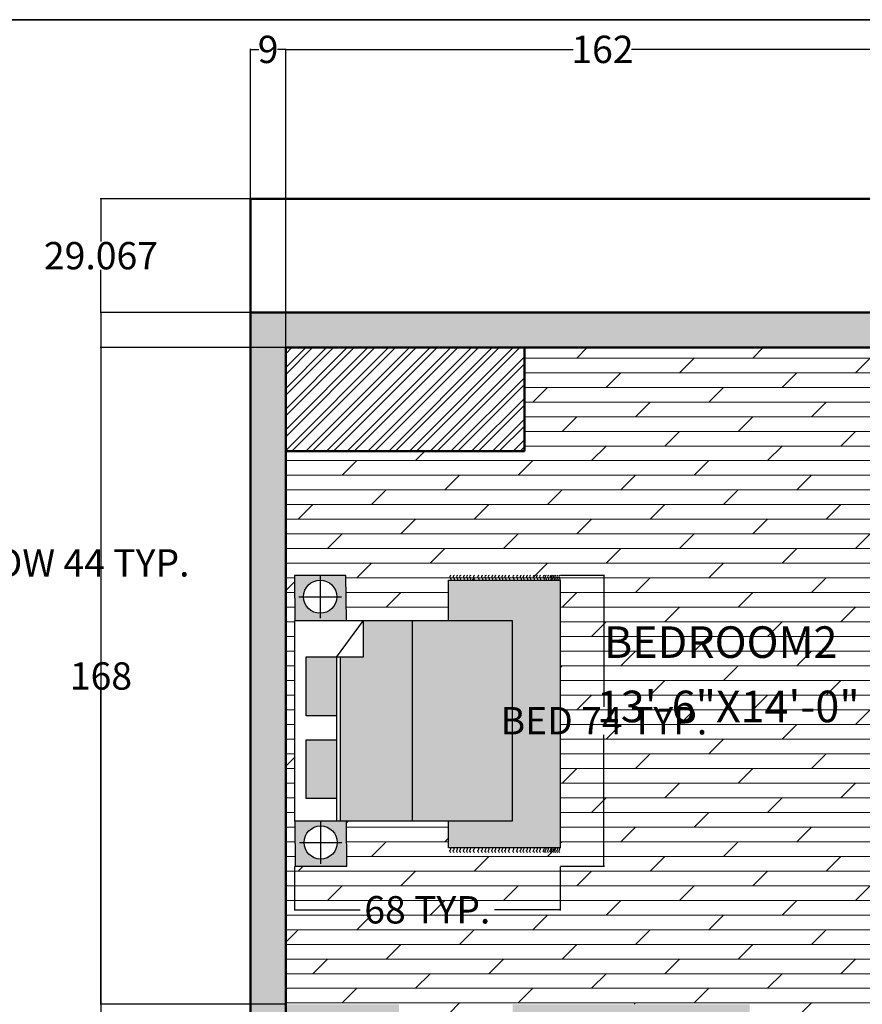
# Model space of a CAD drawing. Units: inches. Extents: x 1381 to 2246, y 1317 to 2168.
# Tile 14 of 15: x 1804 to 2019, y 1916 to 2168. Entities that reach past the tile are written whole.
import ezdxf

# ---------------------------------------------------------------- set-up
doc = ezdxf.new("R2010")
doc.units = ezdxf.units.IN
doc.header["$MEASUREMENT"] = 0
for name, color, linetype, lineweight in [('A-ANNO-DIMS', 2, 'Continuous', 18), ('A-ANNO-TTLB', 7, 'Continuous', 35), ('A-AREA-IDEN', 3, 'Continuous', 25), ('A-FLOR-PATT', 252, 'Continuous', 13), ('A-FURN', 8, 'Continuous', 18), ('A-WALL', 7, 'Continuous', 50), ('A-WALL-PATT', 8, 'Continuous', 13)]:
    doc.layers.add(name, color=color, linetype=linetype, lineweight=lineweight)
doc.layers.add('furniture', color=250, linetype='Continuous')
doc.styles.get("Standard").update_dxf_attribs({"font": 'arial.ttf'})
doc.dimstyles.get("Standard").update_dxf_attribs({"dimtxt": 7, "dimasz": 0.18, "dimexe": 0.18, "dimexo": 0.0625, "dimgap": 0.09, "dimtad": 0, "dimtih": 1, "dimtoh": 1, "dimdec": 1, "dimzin": 0, "dimdsep": 46, "dimlunit": 3, "dimtxsty": 'Standard', "dimcen": 0.09, "dimadec": 0, "dimazin": 0, "dimtfac": 1, "dimtdec": 1, "dimtofl": 0, "dimtmove": 0, "dimatfit": 3, "dimfxl": 1, "dimtolj": 1, "dimtzin": 0, "dimarcsym": 0})

# ---------------------------------------------------------------- blocks, each defined once
blk = doc.blocks.new('CARPET')
at = {"layer": 'furniture'}
for p, q in [((-51.53, -98.11), (-51.53, -55.12)), ((-51.53, -55.12), (-41.27, -55.12)), ((36, -55.12), (51.55, -55.12)), ((51.55, -55.12), (51.55, -98.11)), ((51.55, -98.11), (-51.53, -98.11))]:
    blk.add_line(p, q, dxfattribs=at)
for points, knots in [([(-53.37, -55.99), (-53.22, -55.8), (-52.9, -55.41), (-52.34, -55.8), (-51.89, -56.08), (-51.65, -55.91), (-51.53, -55.83)], [0, 0, 0, 0, 0.653278, 1.290138, 1.740457, 2.114451, 2.114451, 2.114451, 2.114451]), ([(-53.37, -57.26), (-53.22, -57.07), (-52.9, -56.67), (-52.34, -57.07), (-51.89, -57.35), (-51.65, -57.17), (-51.53, -57.1)], [0, 0, 0, 0, 0.653278, 1.290138, 1.740457, 2.114451, 2.114451, 2.114451, 2.114451]), ([(53.37, -55.99), (53.22, -55.8), (52.9, -55.41), (52.34, -55.8), (51.89, -56.08), (51.65, -55.91), (51.53, -55.83)], [0, 0, 0, 0, 0.653278, 1.290138, 1.740457, 2.114451, 2.114451, 2.114451, 2.114451]), ([(53.37, -57.26), (53.22, -57.07), (52.9, -56.67), (52.34, -57.07), (51.89, -57.35), (51.65, -57.17), (51.53, -57.1)], [0, 0, 0, 0, 0.653278, 1.290138, 1.740457, 2.114451, 2.114451, 2.114451, 2.114451]), ([(-53.37, -58.59), (-53.22, -58.4), (-52.9, -58.01), (-52.34, -58.4), (-51.89, -58.68), (-51.65, -58.5), (-51.53, -58.43)], [0, 0, 0, 0, 0.653278, 1.290138, 1.740457, 2.114451, 2.114451, 2.114451, 2.114451]), ([(-53.37, -59.78), (-53.22, -59.58), (-52.9, -59.19), (-52.34, -59.58), (-51.89, -59.86), (-51.65, -59.69), (-51.53, -59.61)], [0, 0, 0, 0, 0.653278, 1.290138, 1.740457, 2.114451, 2.114451, 2.114451, 2.114451]), ([(53.37, -58.59), (53.22, -58.4), (52.9, -58.01), (52.34, -58.4), (51.89, -58.68), (51.65, -58.5), (51.53, -58.43)], [0, 0, 0, 0, 0.653278, 1.290138, 1.740457, 2.114451, 2.114451, 2.114451, 2.114451]), ([(53.37, -59.78), (53.22, -59.58), (52.9, -59.19), (52.34, -59.58), (51.89, -59.86), (51.65, -59.69), (51.53, -59.61)], [0, 0, 0, 0, 0.653278, 1.290138, 1.740457, 2.114451, 2.114451, 2.114451, 2.114451]), ([(-53.37, -61.22), (-53.22, -61.02), (-52.9, -60.63), (-52.34, -61.02), (-51.89, -61.3), (-51.65, -61.13), (-51.53, -61.05)], [0, 0, 0, 0, 0.653278, 1.290138, 1.740457, 2.114451, 2.114451, 2.114451, 2.114451]), ([(-53.37, -62.44), (-53.22, -62.25), (-52.9, -61.86), (-52.34, -62.25), (-51.89, -62.53), (-51.65, -62.36), (-51.53, -62.28)], [0, 0, 0, 0, 0.653278, 1.290138, 1.740457, 2.114451, 2.114451, 2.114451, 2.114451]), ([(-53.37, -63.63), (-53.22, -63.43), (-52.9, -63.04), (-52.34, -63.43), (-51.89, -63.72), (-51.65, -63.54), (-51.53, -63.46)], [0, 0, 0, 0, 0.653278, 1.290138, 1.740457, 2.114451, 2.114451, 2.114451, 2.114451]), ([(53.37, -61.22), (53.22, -61.02), (52.9, -60.63), (52.34, -61.02), (51.89, -61.3), (51.65, -61.13), (51.53, -61.05)], [0, 0, 0, 0, 0.653278, 1.290138, 1.740457, 2.114451, 2.114451, 2.114451, 2.114451]), ([(53.37, -62.44), (53.22, -62.25), (52.9, -61.86), (52.34, -62.25), (51.89, -62.53), (51.65, -62.36), (51.53, -62.28)], [0, 0, 0, 0, 0.653278, 1.290138, 1.740457, 2.114451, 2.114451, 2.114451, 2.114451]), ([(53.37, -63.63), (53.22, -63.43), (52.9, -63.04), (52.34, -63.43), (51.89, -63.72), (51.65, -63.54), (51.53, -63.46)], [0, 0, 0, 0, 0.653278, 1.290138, 1.740457, 2.114451, 2.114451, 2.114451, 2.114451]), ([(-53.37, -65.07), (-53.22, -64.87), (-52.9, -64.48), (-52.34, -64.87), (-51.89, -65.15), (-51.65, -64.98), (-51.53, -64.9)], [0, 0, 0, 0, 0.653278, 1.290138, 1.740457, 2.114451, 2.114451, 2.114451, 2.114451]), ([(-53.37, -66.76), (-53.22, -66.56), (-52.9, -66.17), (-52.34, -66.56), (-51.89, -66.84), (-51.65, -66.67), (-51.53, -66.59)], [0, 0, 0, 0, 0.653278, 1.290138, 1.740457, 2.114451, 2.114451, 2.114451, 2.114451]), ([(-53.37, -68.2), (-53.22, -68), (-52.9, -67.61), (-52.34, -68), (-51.89, -68.28), (-51.65, -68.11), (-51.53, -68.03)], [0, 0, 0, 0, 0.653278, 1.290138, 1.740457, 2.114451, 2.114451, 2.114451, 2.114451]), ([(53.37, -65.07), (53.22, -64.87), (52.9, -64.48), (52.34, -64.87), (51.89, -65.15), (51.65, -64.98), (51.53, -64.9)], [0, 0, 0, 0, 0.653278, 1.290138, 1.740457, 2.114451, 2.114451, 2.114451, 2.114451]), ([(53.37, -66.76), (53.22, -66.56), (52.9, -66.17), (52.34, -66.56), (51.89, -66.84), (51.65, -66.67), (51.53, -66.59)], [0, 0, 0, 0, 0.653278, 1.290138, 1.740457, 2.114451, 2.114451, 2.114451, 2.114451]), ([(53.37, -68.2), (53.22, -68), (52.9, -67.61), (52.34, -68), (51.89, -68.28), (51.65, -68.11), (51.53, -68.03)], [0, 0, 0, 0, 0.653278, 1.290138, 1.740457, 2.114451, 2.114451, 2.114451, 2.114451]), ([(-53.37, -69.53), (-53.22, -69.33), (-52.9, -68.94), (-52.34, -69.33), (-51.89, -69.61), (-51.65, -69.44), (-51.53, -69.36)], [0, 0, 0, 0, 0.653278, 1.290138, 1.740457, 2.114451, 2.114451, 2.114451, 2.114451]), ([(-53.37, -70.79), (-53.22, -70.6), (-52.9, -70.21), (-52.34, -70.6), (-51.89, -70.88), (-51.65, -70.7), (-51.53, -70.63)], [0, 0, 0, 0, 0.653278, 1.290138, 1.740457, 2.114451, 2.114451, 2.114451, 2.114451]), ([(-53.37, -72.12), (-53.22, -71.93), (-52.9, -71.54), (-52.34, -71.93), (-51.89, -72.21), (-51.65, -72.04), (-51.53, -71.96)], [0, 0, 0, 0, 0.653278, 1.290138, 1.740457, 2.114451, 2.114451, 2.114451, 2.114451]), ([(53.37, -69.53), (53.22, -69.33), (52.9, -68.94), (52.34, -69.33), (51.89, -69.61), (51.65, -69.44), (51.53, -69.36)], [0, 0, 0, 0, 0.653278, 1.290138, 1.740457, 2.114451, 2.114451, 2.114451, 2.114451]), ([(53.37, -70.79), (53.22, -70.6), (52.9, -70.21), (52.34, -70.6), (51.89, -70.88), (51.65, -70.7), (51.53, -70.63)], [0, 0, 0, 0, 0.653278, 1.290138, 1.740457, 2.114451, 2.114451, 2.114451, 2.114451]), ([(53.37, -72.12), (53.22, -71.93), (52.9, -71.54), (52.34, -71.93), (51.89, -72.21), (51.65, -72.04), (51.53, -71.96)], [0, 0, 0, 0, 0.653278, 1.290138, 1.740457, 2.114451, 2.114451, 2.114451, 2.114451]), ([(-53.37, -73.31), (-53.22, -73.11), (-52.9, -72.72), (-52.34, -73.11), (-51.89, -73.4), (-51.65, -73.22), (-51.53, -73.14)], [0, 0, 0, 0, 0.653278, 1.290138, 1.740457, 2.114451, 2.114451, 2.114451, 2.114451]), ([(-53.37, -74.75), (-53.22, -74.55), (-52.9, -74.16), (-52.34, -74.55), (-51.89, -74.83), (-51.65, -74.66), (-51.53, -74.58)], [0, 0, 0, 0, 0.653278, 1.290138, 1.740457, 2.114451, 2.114451, 2.114451, 2.114451]), ([(-53.37, -75.98), (-53.22, -75.78), (-52.9, -75.39), (-52.34, -75.78), (-51.89, -76.06), (-51.65, -75.89), (-51.53, -75.81)], [0, 0, 0, 0, 0.653278, 1.290138, 1.740457, 2.114451, 2.114451, 2.114451, 2.114451]), ([(53.37, -73.31), (53.22, -73.11), (52.9, -72.72), (52.34, -73.11), (51.89, -73.4), (51.65, -73.22), (51.53, -73.14)], [0, 0, 0, 0, 0.653278, 1.290138, 1.740457, 2.114451, 2.114451, 2.114451, 2.114451]), ([(53.37, -74.75), (53.22, -74.55), (52.9, -74.16), (52.34, -74.55), (51.89, -74.83), (51.65, -74.66), (51.53, -74.58)], [0, 0, 0, 0, 0.653278, 1.290138, 1.740457, 2.114451, 2.114451, 2.114451, 2.114451]), ([(53.37, -75.98), (53.22, -75.78), (52.9, -75.39), (52.34, -75.78), (51.89, -76.06), (51.65, -75.89), (51.53, -75.81)], [0, 0, 0, 0, 0.653278, 1.290138, 1.740457, 2.114451, 2.114451, 2.114451, 2.114451]), ([(-53.37, -77.16), (-53.22, -76.96), (-52.9, -76.57), (-52.34, -76.96), (-51.89, -77.25), (-51.65, -77.07), (-51.53, -76.99)], [0, 0, 0, 0, 0.653278, 1.290138, 1.740457, 2.114451, 2.114451, 2.114451, 2.114451]), ([(-53.37, -78.6), (-53.22, -78.4), (-52.9, -78.01), (-52.34, -78.4), (-51.89, -78.68), (-51.65, -78.51), (-51.53, -78.43)], [0, 0, 0, 0, 0.653278, 1.290138, 1.740457, 2.114451, 2.114451, 2.114451, 2.114451]), ([(53.37, -77.16), (53.22, -76.96), (52.9, -76.57), (52.34, -76.96), (51.89, -77.25), (51.65, -77.07), (51.53, -76.99)], [0, 0, 0, 0, 0.653278, 1.290138, 1.740457, 2.114451, 2.114451, 2.114451, 2.114451]), ([(53.37, -78.6), (53.22, -78.4), (52.9, -78.01), (52.34, -78.4), (51.89, -78.68), (51.65, -78.51), (51.53, -78.43)], [0, 0, 0, 0, 0.653278, 1.290138, 1.740457, 2.114451, 2.114451, 2.114451, 2.114451]), ([(-53.37, -80.29), (-53.22, -80.09), (-52.9, -79.7), (-52.34, -80.09), (-51.89, -80.37), (-51.65, -80.2), (-51.53, -80.12)], [0, 0, 0, 0, 0.653278, 1.290138, 1.740457, 2.114451, 2.114451, 2.114451, 2.114451]), ([(-53.37, -81.73), (-53.22, -81.53), (-52.9, -81.14), (-52.34, -81.53), (-51.89, -81.81), (-51.65, -81.64), (-51.53, -81.56)], [0, 0, 0, 0, 0.653278, 1.290138, 1.740457, 2.114451, 2.114451, 2.114451, 2.114451]), ([(-53.37, -83.06), (-53.22, -82.86), (-52.9, -82.47), (-52.34, -82.86), (-51.89, -83.14), (-51.65, -82.97), (-51.53, -82.89)], [0, 0, 0, 0, 0.653278, 1.290138, 1.740457, 2.114451, 2.114451, 2.114451, 2.114451]), ([(53.37, -80.29), (53.22, -80.09), (52.9, -79.7), (52.34, -80.09), (51.89, -80.37), (51.65, -80.2), (51.53, -80.12)], [0, 0, 0, 0, 0.653278, 1.290138, 1.740457, 2.114451, 2.114451, 2.114451, 2.114451]), ([(53.37, -81.73), (53.22, -81.53), (52.9, -81.14), (52.34, -81.53), (51.89, -81.81), (51.65, -81.64), (51.53, -81.56)], [0, 0, 0, 0, 0.653278, 1.290138, 1.740457, 2.114451, 2.114451, 2.114451, 2.114451]), ([(53.37, -83.06), (53.22, -82.86), (52.9, -82.47), (52.34, -82.86), (51.89, -83.14), (51.65, -82.97), (51.53, -82.89)], [0, 0, 0, 0, 0.653278, 1.290138, 1.740457, 2.114451, 2.114451, 2.114451, 2.114451]), ([(-53.37, -84.18), (-53.22, -83.99), (-52.9, -83.6), (-52.34, -83.99), (-51.89, -84.27), (-51.65, -84.09), (-51.53, -84.02)], [0, 0, 0, 0, 0.653278, 1.290138, 1.740457, 2.114451, 2.114451, 2.114451, 2.114451]), ([(-53.37, -85.51), (-53.22, -85.32), (-52.9, -84.93), (-52.34, -85.32), (-51.89, -85.6), (-51.65, -85.42), (-51.53, -85.35)], [0, 0, 0, 0, 0.653278, 1.290138, 1.740457, 2.114451, 2.114451, 2.114451, 2.114451]), ([(-53.37, -86.7), (-53.22, -86.5), (-52.9, -86.11), (-52.34, -86.5), (-51.89, -86.78), (-51.65, -86.61), (-51.53, -86.53)], [0, 0, 0, 0, 0.653278, 1.290138, 1.740457, 2.114451, 2.114451, 2.114451, 2.114451]), ([(53.37, -84.18), (53.22, -83.99), (52.9, -83.6), (52.34, -83.99), (51.89, -84.27), (51.65, -84.09), (51.53, -84.02)], [0, 0, 0, 0, 0.653278, 1.290138, 1.740457, 2.114451, 2.114451, 2.114451, 2.114451]), ([(53.37, -85.51), (53.22, -85.32), (52.9, -84.93), (52.34, -85.32), (51.89, -85.6), (51.65, -85.42), (51.53, -85.35)], [0, 0, 0, 0, 0.653278, 1.290138, 1.740457, 2.114451, 2.114451, 2.114451, 2.114451]), ([(53.37, -86.7), (53.22, -86.5), (52.9, -86.11), (52.34, -86.5), (51.89, -86.78), (51.65, -86.61), (51.53, -86.53)], [0, 0, 0, 0, 0.653278, 1.290138, 1.740457, 2.114451, 2.114451, 2.114451, 2.114451]), ([(-53.37, -88.14), (-53.22, -87.94), (-52.9, -87.55), (-52.34, -87.94), (-51.89, -88.22), (-51.65, -88.05), (-51.53, -87.97)], [0, 0, 0, 0, 0.653278, 1.290138, 1.740457, 2.114451, 2.114451, 2.114451, 2.114451]), ([(-53.37, -89.36), (-53.22, -89.17), (-52.9, -88.78), (-52.34, -89.17), (-51.89, -89.45), (-51.65, -89.28), (-51.53, -89.2)], [0, 0, 0, 0, 0.653278, 1.290138, 1.740457, 2.114451, 2.114451, 2.114451, 2.114451]), ([(-53.37, -90.55), (-53.22, -90.35), (-52.9, -89.96), (-52.34, -90.35), (-51.89, -90.64), (-51.65, -90.46), (-51.53, -90.38)], [0, 0, 0, 0, 0.653278, 1.290138, 1.740457, 2.114451, 2.114451, 2.114451, 2.114451]), ([(53.37, -88.14), (53.22, -87.94), (52.9, -87.55), (52.34, -87.94), (51.89, -88.22), (51.65, -88.05), (51.53, -87.97)], [0, 0, 0, 0, 0.653278, 1.290138, 1.740457, 2.114451, 2.114451, 2.114451, 2.114451]), ([(53.37, -89.36), (53.22, -89.17), (52.9, -88.78), (52.34, -89.17), (51.89, -89.45), (51.65, -89.28), (51.53, -89.2)], [0, 0, 0, 0, 0.653278, 1.290138, 1.740457, 2.114451, 2.114451, 2.114451, 2.114451]), ([(53.37, -90.55), (53.22, -90.35), (52.9, -89.96), (52.34, -90.35), (51.9, -90.63), (51.66, -90.47), (51.55, -90.4)], [0, 0, 0, 0, 0.653278, 1.290138, 1.740457, 2.0926, 2.0926, 2.0926, 2.0926]), ([(-53.37, -91.99), (-53.22, -91.79), (-52.9, -91.4), (-52.34, -91.79), (-51.89, -92.07), (-51.65, -91.9), (-51.53, -91.82)], [0, 0, 0, 0, 0.653278, 1.290138, 1.740457, 2.114451, 2.114451, 2.114451, 2.114451]), ([(-53.37, -92.69), (-53.22, -92.48), (-52.9, -92.08), (-52.35, -92.49), (-51.89, -92.77), (-51.65, -92.6), (-51.53, -92.52)], [0, 0, 0, 0, 0.663904, 1.307406, 1.757725, 2.131719, 2.131719, 2.131719, 2.131719]), ([(-53.37, -93.61), (-53.22, -93.42), (-52.9, -93.03), (-52.34, -93.42), (-51.89, -93.7), (-51.65, -93.52), (-51.53, -93.45)], [0, 0, 0, 0, 0.653278, 1.290138, 1.740457, 2.114451, 2.114451, 2.114451, 2.114451]), ([(-53.37, -94.55), (-53.22, -94.35), (-52.9, -93.96), (-52.34, -94.35), (-51.89, -94.63), (-51.65, -94.46), (-51.53, -94.38)], [0, 0, 0, 0, 0.653278, 1.290138, 1.740457, 2.114451, 2.114451, 2.114451, 2.114451]), ([(-53.37, -95.05), (-53.22, -94.85), (-52.9, -94.46), (-52.34, -94.85), (-51.89, -95.14), (-51.65, -94.96), (-51.53, -94.88)], [0, 0, 0, 0, 0.653278, 1.290138, 1.740457, 2.114451, 2.114451, 2.114451, 2.114451]), ([(53.37, -91.99), (53.22, -91.79), (52.9, -91.4), (52.34, -91.79), (51.9, -92.07), (51.66, -91.91), (51.55, -91.83)], [0, 0, 0, 0, 0.653278, 1.290138, 1.740457, 2.0926, 2.0926, 2.0926, 2.0926]), ([(53.37, -92.69), (53.22, -92.49), (52.9, -92.09), (52.34, -92.49), (51.9, -92.77), (51.66, -92.61), (51.55, -92.53)], [0, 0, 0, 0, 0.656792, 1.295826, 1.746145, 2.098292, 2.098292, 2.098292, 2.098292]), ([(53.37, -93.66), (53.22, -93.46), (52.9, -93.07), (52.34, -93.46), (51.9, -93.74), (51.66, -93.58), (51.55, -93.5)], [0, 0, 0, 0, 0.653278, 1.290138, 1.740457, 2.0926, 2.0926, 2.0926, 2.0926]), ([(53.37, -94.59), (53.22, -94.4), (52.9, -94.01), (52.34, -94.4), (51.9, -94.68), (51.66, -94.51), (51.55, -94.44)], [0, 0, 0, 0, 0.653278, 1.290138, 1.740457, 2.0926, 2.0926, 2.0926, 2.0926]), ([(53.37, -95.1), (53.22, -94.9), (52.9, -94.51), (52.34, -94.9), (51.9, -95.18), (51.66, -95.02), (51.55, -94.94)], [0, 0, 0, 0, 0.653278, 1.290138, 1.740457, 2.0926, 2.0926, 2.0926, 2.0926]), ([(-53.37, -95.73), (-53.22, -95.54), (-52.9, -95.15), (-52.34, -95.54), (-51.89, -95.82), (-51.65, -95.65), (-51.53, -95.57)], [0, 0, 0, 0, 0.653278, 1.290138, 1.740457, 2.114451, 2.114451, 2.114451, 2.114451]), ([(-53.37, -96.38), (-53.22, -96.18), (-52.9, -95.79), (-52.34, -96.18), (-51.89, -96.47), (-51.65, -96.29), (-51.53, -96.21)], [0, 0, 0, 0, 0.653278, 1.290138, 1.740457, 2.114451, 2.114451, 2.114451, 2.114451]), ([(-53.37, -97.17), (-53.22, -96.98), (-52.9, -96.59), (-52.34, -96.98), (-51.89, -97.26), (-51.65, -97.08), (-51.53, -97.01)], [0, 0, 0, 0, 0.653278, 1.290138, 1.740457, 2.114451, 2.114451, 2.114451, 2.114451]), ([(-53.37, -97.99), (-53.22, -97.79), (-52.9, -97.4), (-52.34, -97.79), (-51.89, -98.08), (-51.65, -97.9), (-51.53, -97.82)], [0, 0, 0, 0, 0.653278, 1.290138, 1.740457, 2.114451, 2.114451, 2.114451, 2.114451]), ([(53.37, -95.78), (53.22, -95.58), (52.9, -95.19), (52.34, -95.58), (51.89, -95.86), (51.65, -95.69), (51.53, -95.61)], [0, 0, 0, 0, 0.653278, 1.290138, 1.740457, 2.114451, 2.114451, 2.114451, 2.114451]), ([(53.37, -96.43), (53.22, -96.23), (52.9, -95.84), (52.34, -96.23), (51.89, -96.51), (51.65, -96.34), (51.53, -96.26)], [0, 0, 0, 0, 0.653278, 1.290138, 1.740457, 2.114451, 2.114451, 2.114451, 2.114451]), ([(53.37, -97.22), (53.22, -97.02), (52.9, -96.63), (52.34, -97.02), (51.89, -97.3), (51.65, -97.13), (51.53, -97.05)], [0, 0, 0, 0, 0.653278, 1.290138, 1.740457, 2.114451, 2.114451, 2.114451, 2.114451]), ([(53.37, -97.99), (53.22, -97.79), (52.9, -97.4), (52.34, -97.79), (51.89, -98.08), (51.65, -97.9), (51.53, -97.82)], [0, 0, 0, 0, 0.653278, 1.290138, 1.740457, 2.114451, 2.114451, 2.114451, 2.114451])]:
    blk.add_open_spline(points, degree=3, knots=knots, dxfattribs=at)
blk = doc.blocks.new('A$C58D270C6')
at = {"layer": 'furniture'}
for p, q in [((9.09, 124.13), (9.09, 108.87)), ((1.46, 116.5), (16.73, 116.5)), ((14.97, 94.84), (24.62, 107.92)), ((24.62, 94.93), (24.62, 107.92)), ((42.08, 108), (42.08, 36)), ((14.97, 94.93), (24.62, 94.93)), ((14.97, 94.84), (14.97, 36)), ((16.22, 94.93), (16.22, 36)), ((9.25, 36), (9.25, 20.74)), ((1.62, 28.37), (16.88, 28.37))]:
    blk.add_line(p, q, dxfattribs=at)
for points in [[(18.5, 108), (18.34, 124.13), (-0.16, 124.13), (0, 108)], [(0, 108), (77.91, 108), (77.91, 36), (0, 36)], [(4.09, 94.93), (14.97, 94.93), (14.97, 73.83), (4.09, 73.83)], [(4.09, 65.23), (14.97, 65.23), (14.97, 44.13), (4.09, 44.13)], [(18.65, 19.87), (18.5, 36), (0, 36), (0.16, 19.87)]]:
    blk.add_lwpolyline(points, close=True, dxfattribs=at)
for centre in [(9.09, 116.5), (9.25, 28.37)]:
    blk.add_circle(centre, 5.95, dxfattribs=at)
at = {"layer": 'furniture', "xscale": 0.9312884925094044, "yscale": 0.9312884925094044, "zscale": 0.9312884925094044, "rotation": 90}
blk.add_blockref('CARPET', (3.79, 74.47), dxfattribs=at)
blk = doc.blocks.new('*D21')
at = {"layer": 'A-ANNO-DIMS', "color": 0, "lineweight": -2, "transparency": 16777216}
for p, q in [((1942.08, 2025.67), (1953.36, 2025.67)), ((1953.18, 2025.49), (1953.18, 1992.06)), ((1953.18, 1951.44), (1953.18, 1984.87)), ((1942.08, 1951.26), (1953.36, 1951.26))]:
    blk.add_line(p, q, dxfattribs=at)
at = {"layer": 'A-ANNO-DIMS', "color": 0, "transparency": 16777216}
for points in [[(1953.15, 2025.49), (1953.21, 2025.49), (1953.18, 2025.67)], [(1953.15, 1951.44), (1953.21, 1951.44), (1953.18, 1951.26)]]:
    blk.add_solid(points, dxfattribs=at)
at = {"layer": 'Defpoints', "color": 0, "transparency": 16777216}
for p in [(1942.02, 2025.67), (1953.18, 2025.67), (1942.02, 1951.26)]:
    blk.add_point(p, dxfattribs=at)
at = {"layer": 'A-ANNO-DIMS', "color": 0, "transparency": 16777216, "insert": (1953.18, 1988.47), "char_height": 7, "attachment_point": 5}
blk.add_mtext('\\A1;BED 74 TYP.', dxfattribs=at)
blk = doc.blocks.new('*D22')
at = {"layer": 'A-ANNO-DIMS', "color": 0, "lineweight": -2, "transparency": 16777216}
for p, q in [((1874.03, 1951.2), (1874.03, 1939.92)), ((1942.02, 1951.2), (1942.02, 1939.92)), ((1874.21, 1940.1), (1890.88, 1940.1)), ((1941.84, 1940.1), (1925.17, 1940.1))]:
    blk.add_line(p, q, dxfattribs=at)
at = {"layer": 'A-ANNO-DIMS', "color": 0, "transparency": 16777216}
for points in [[(1874.21, 1940.13), (1874.21, 1940.07), (1874.03, 1940.1)], [(1941.84, 1940.13), (1941.84, 1940.07), (1942.02, 1940.1)]]:
    blk.add_solid(points, dxfattribs=at)
at = {"layer": 'Defpoints', "color": 0, "transparency": 16777216}
for p in [(1874.03, 1951.26), (1942.02, 1951.26), (1942.02, 1940.1)]:
    blk.add_point(p, dxfattribs=at)
at = {"layer": 'A-ANNO-DIMS', "color": 0, "transparency": 16777216, "insert": (1908.02, 1940.1), "char_height": 7, "attachment_point": 5}
blk.add_mtext('\\A1;68 TYP.', dxfattribs=at)
blk = doc.blocks.new('*D41')
at = {"layer": 'A-ANNO-DIMS', "color": 0, "lineweight": -2, "transparency": 16777216}
for p, q in [((1682.28, 2035.35), (1682.28, 2028.68)), ((1725.96, 2035.35), (1725.96, 2028.68)), ((1682.46, 2028.86), (1725.78, 2028.86)), ((1725.96, 2028.86), (1726.14, 2028.86))]:
    blk.add_line(p, q, dxfattribs=at)
at = {"layer": 'A-ANNO-DIMS', "color": 0, "transparency": 16777216}
for points in [[(1682.46, 2028.89), (1682.46, 2028.83), (1682.28, 2028.86)], [(1725.78, 2028.89), (1725.78, 2028.83), (1725.96, 2028.86)]]:
    blk.add_solid(points, dxfattribs=at)
at = {"layer": 'Defpoints', "color": 0, "transparency": 16777216}
for p in [(1682.28, 2035.42), (1725.96, 2035.42), (1725.96, 2028.86)]:
    blk.add_point(p, dxfattribs=at)
at = {"layer": 'A-ANNO-DIMS', "color": 0, "transparency": 16777216, "insert": (1788.75, 2028.86), "char_height": 7, "attachment_point": 5}
blk.add_mtext('\\A1;KITCHEN WINDOW 44 TYP.', dxfattribs=at)
blk = doc.blocks.new('*D76')
at = {"layer": 'A-ANNO-DIMS', "color": 0, "lineweight": -2, "transparency": 16777216}
for p, q in [((1862.74, 2092.92), (1824.38, 2092.92)), ((1824.56, 2092.74), (1824.56, 1786.08)), ((1824.56, 1472.1), (1824.56, 1778.75)), ((1862.74, 1471.92), (1824.38, 1471.92))]:
    blk.add_line(p, q, dxfattribs=at)
at = {"layer": 'A-ANNO-DIMS', "color": 0, "transparency": 16777216}
for points in [[(1824.53, 2092.74), (1824.59, 2092.74), (1824.56, 2092.92)], [(1824.53, 1472.1), (1824.59, 1472.1), (1824.56, 1471.92)]]:
    blk.add_solid(points, dxfattribs=at)
at = {"layer": 'Defpoints', "color": 0, "transparency": 16777216}
for p in [(1824.56, 2092.92), (1862.81, 2092.92), (1862.81, 1471.92)]:
    blk.add_point(p, dxfattribs=at)
at = {"layer": 'A-ANNO-DIMS', "color": 0, "transparency": 16777216, "insert": (1824.56, 1782.42), "char_height": 7, "attachment_point": 5}
blk.add_mtext('\\A1;621', dxfattribs=at)
blk = doc.blocks.new('*D77')
at = {"layer": 'A-ANNO-DIMS', "color": 0, "lineweight": -2, "transparency": 16777216}
for p, q in [((1862.74, 2121.98), (1824.38, 2121.98)), ((1824.56, 2121.8), (1824.56, 2111.11)), ((1824.56, 2093.1), (1824.56, 2103.79)), ((1862.74, 2092.92), (1824.38, 2092.92))]:
    blk.add_line(p, q, dxfattribs=at)
at = {"layer": 'A-ANNO-DIMS', "color": 0, "transparency": 16777216}
for points in [[(1824.53, 2121.8), (1824.59, 2121.8), (1824.56, 2121.98)], [(1824.53, 2093.1), (1824.59, 2093.1), (1824.56, 2092.92)]]:
    blk.add_solid(points, dxfattribs=at)
at = {"layer": 'Defpoints', "color": 0, "transparency": 16777216}
for p in [(1824.56, 2121.98), (1862.81, 2121.98), (1862.81, 2092.92)]:
    blk.add_point(p, dxfattribs=at)
at = {"layer": 'A-ANNO-DIMS', "color": 0, "transparency": 16777216, "insert": (1824.56, 2107.45), "char_height": 7, "attachment_point": 5}
blk.add_mtext('\\A1;29.067', dxfattribs=at)
blk = doc.blocks.new('*D79')
at = {"layer": 'A-ANNO-DIMS', "color": 0, "lineweight": -2, "transparency": 16777216}
for p, q in [((1862.81, 2092.98), (1862.81, 2160.41)), ((1862.99, 2160.23), (1864.91, 2160.23)), ((1871.63, 2160.23), (1869.7, 2160.23)), ((1871.81, 2083.98), (1871.81, 2160.41))]:
    blk.add_line(p, q, dxfattribs=at)
at = {"layer": 'A-ANNO-DIMS', "color": 0, "transparency": 16777216}
for points in [[(1862.99, 2160.26), (1862.99, 2160.2), (1862.81, 2160.23)], [(1871.63, 2160.26), (1871.63, 2160.2), (1871.81, 2160.23)]]:
    blk.add_solid(points, dxfattribs=at)
at = {"layer": 'Defpoints', "color": 0, "transparency": 16777216}
for p in [(1871.81, 2160.23), (1862.81, 2092.92), (1871.81, 2083.92)]:
    blk.add_point(p, dxfattribs=at)
at = {"layer": 'A-ANNO-DIMS', "color": 0, "transparency": 16777216, "insert": (1867.31, 2160.23), "char_height": 7, "attachment_point": 5}
blk.add_mtext('\\A1;9', dxfattribs=at)
blk = doc.blocks.new('*D83')
at = {"layer": 'A-ANNO-DIMS', "color": 0, "lineweight": -2, "transparency": 16777216}
for p, q in [((1871.74, 2083.92), (1824.38, 2083.92)), ((1824.56, 2083.74), (1824.56, 2003.58)), ((1824.56, 1916.1), (1824.56, 1996.25)), ((1871.74, 1915.92), (1824.38, 1915.92))]:
    blk.add_line(p, q, dxfattribs=at)
at = {"layer": 'A-ANNO-DIMS', "color": 0, "transparency": 16777216}
for points in [[(1824.53, 2083.74), (1824.59, 2083.74), (1824.56, 2083.92)], [(1824.53, 1916.1), (1824.59, 1916.1), (1824.56, 1915.92)]]:
    blk.add_solid(points, dxfattribs=at)
at = {"layer": 'Defpoints', "color": 0, "transparency": 16777216}
for p in [(1824.56, 2083.92), (1871.81, 2083.92), (1871.81, 1915.92)]:
    blk.add_point(p, dxfattribs=at)
at = {"layer": 'A-ANNO-DIMS', "color": 0, "transparency": 16777216, "insert": (1824.56, 1999.92), "char_height": 7, "attachment_point": 5}
blk.add_mtext('\\A1;168', dxfattribs=at)
blk = doc.blocks.new('*D84')
at = {"layer": 'A-ANNO-DIMS', "color": 0, "lineweight": -2, "transparency": 16777216}
for p, q in [((1871.81, 2083.98), (1871.81, 2160.41)), ((1871.99, 2160.23), (1945.35, 2160.23)), ((2033.63, 2160.23), (1960.26, 2160.23)), ((2033.81, 2083.98), (2033.81, 2160.41))]:
    blk.add_line(p, q, dxfattribs=at)
at = {"layer": 'A-ANNO-DIMS', "color": 0, "transparency": 16777216}
for points in [[(1871.99, 2160.26), (1871.99, 2160.2), (1871.81, 2160.23)], [(2033.63, 2160.26), (2033.63, 2160.2), (2033.81, 2160.23)]]:
    blk.add_solid(points, dxfattribs=at)
at = {"layer": 'Defpoints', "color": 0, "transparency": 16777216}
for p in [(2033.81, 2160.23), (1871.81, 2083.92), (2033.81, 2083.92)]:
    blk.add_point(p, dxfattribs=at)
at = {"layer": 'A-ANNO-DIMS', "color": 0, "transparency": 16777216, "insert": (1952.81, 2160.23), "char_height": 7, "attachment_point": 5}
blk.add_mtext('\\A1;162', dxfattribs=at)

msp = doc.modelspace()

# ---------------------------------------------------------------- hatches: boundary and pattern name
at = {"layer": 'A-FLOR-PATT'}
h = msp.add_hatch(dxfattribs=at)
h.set_pattern_fill('ANSI32', color=256, scale=10)
h.set_pattern_definition([(45, (415.7542, 373.5), (-2.6516504, 2.6516504), []), (45, (417.522, 373.5), (-2.6516504, 2.6516504), [])])
h.paths.add_polyline_path([(1932.8736, 2083.9163), (1871.8052, 2083.9163), (1871.8052, 2057.4148), (1932.8736, 2057.4148)])
h = msp.add_hatch(dxfattribs=at)
h.set_pattern_fill('DOLMIT', color=256, scale=15)
h.paths.add_polyline_path([(2033.8052, 2083.9163), (1932.8359, 2083.9163), (1932.8359, 2057.4148), (1871.8052, 2057.4148), (1871.8052, 1915.9163), (1900.7902, 1915.9163), (1900.7902, 1913.6663), (1929.807, 1913.6663), (1929.807, 1915.9163), (1990.4785, 1915.9163), (1990.4785, 1913.6663), (2028.7731, 1913.6663), (2028.7731, 1915.9163), (2033.8052, 1915.9163)])
edge = h.paths.add_edge_path(flags=16)
edge.add_spline(control_points=[(1939.5401, 1955.9789), (1939.5923, 1955.9054), (1939.7074, 1955.7434), (1939.52, 1955.4418), (1939.2609, 1955.0703), (1939.5201, 1954.8623), (1939.6513, 1954.757)], knot_values=[0, 0, 0, 0, 0.37399428, 0.82431366, 1.46117297, 2.11445126, 2.11445126, 2.11445126, 2.11445126], degree=3, periodic=0)
edge.add_spline(control_points=[(1939.8748, 1955.9789), (1939.9271, 1955.9054), (1940.0422, 1955.7434), (1939.8548, 1955.4418), (1939.5956, 1955.0703), (1939.8548, 1954.8623), (1939.986, 1954.757)], knot_values=[0, 0, 0, 0, 0.37399428, 0.82431366, 1.46117297, 2.11445126, 2.11445126, 2.11445126, 2.11445126], degree=3, periodic=0)
edge = h.paths.add_edge_path(flags=16)
edge.add_line((1942.0171, 2024.4608), (1942.0171, 1955.9789))
edge.add_line((1942.0171, 1955.9789), (1913.4617, 1955.9789))
edge.add_line((1913.4617, 1955.9789), (1913.4617, 1962.7697))
edge.add_line((1913.4617, 1962.7697), (1887.334, 1962.7697))
edge.add_line((1887.334, 1962.7697), (1887.445, 1951.263))
edge.add_line((1887.445, 1951.263), (1874.2492, 1951.263))
edge.add_line((1874.2492, 1951.263), (1874.1382, 1962.7697))
edge.add_line((1874.1382, 1962.7697), (1874.1382, 2014.1291))
edge.add_line((1874.1382, 2014.1291), (1874.0273, 2025.6358))
edge.add_line((1874.0273, 2025.6358), (1887.2231, 2025.6358))
edge.add_line((1887.2231, 2025.6358), (1887.334, 2014.1291))
edge.add_line((1887.334, 2014.1291), (1913.4617, 2014.1291))
edge.add_line((1913.4617, 2014.1291), (1913.4617, 2024.4608))
edge.add_line((1913.4617, 2024.4608), (1939.579, 2024.4608))
edge.add_spline(control_points=[(1939.579, 2024.4608), (1939.6269, 2024.5305), (1939.736, 2024.6891), (1939.5499, 2024.9858), (1939.2914, 2025.3575), (1939.5505, 2025.5655), (1939.6817, 2025.6708)], knot_values=[0, 0, 0, 0, 0.3521435, 0.80246288, 1.43932219, 2.09260048, 2.09260048, 2.09260048, 2.09260048], degree=3, periodic=0)
edge.add_spline(control_points=[(1940.0164, 2025.6708), (1939.8852, 2025.5655), (1939.6261, 2025.3575), (1939.8847, 2024.9858), (1940.0707, 2024.6891), (1939.9616, 2024.5305), (1939.9137, 2024.4608)], knot_values=[0, 0, 0, 0, 0.65327829, 1.2901376, 1.74045698, 2.09260048, 2.09260048, 2.09260048, 2.09260048], degree=3, periodic=0)
edge.add_line((1939.9137, 2024.4608), (1942.0171, 2024.4608))
h.paths.add_polyline_path([(1891.698, 2014.0737), (1891.698, 2004.8072), (1884.8656, 2004.8072), (1884.8197, 2004.7449), (1884.8197, 1968.5691), (1877.0588, 1968.5691), (1877.0588, 1983.6181), (1884.8197, 1983.6181), (1884.8197, 1989.7582), (1877.0588, 1989.7582), (1877.0588, 2004.8072), (1884.8656, 2004.8072)], flags=0)
h.paths.add_polyline_path([(1884.8729, 2020.1923, -1), (1876.3774, 2020.1923, -1)], flags=0)
h.paths.add_polyline_path([(1884.9838, 1957.3262, -1), (1876.4884, 1957.3262, -1)], flags=0)
h.paths.add_polyline_path([(1949.3287, 1985.8776), (2018.4467, 1985.8776), (2018.4467, 1998.2538), (1949.3287, 1998.2538)], flags=24)
h.paths.add_polyline_path([(1951.1032, 2002.3157), (2019.8384, 2002.3157), (2019.8384, 2014.8488), (1951.1032, 2014.8488)], flags=24)
at = {"layer": 'A-FURN'}
h = msp.add_hatch(color=256, dxfattribs=at)
h.dxf.hatch_style = 1
h.paths.add_polyline_path([(1876.3774, 2020.1923, -0.41421356), (1880.6252, 2024.44), (1880.6252, 2025.6358), (1874.0273, 2025.6358), (1874.1382, 2014.1291), (1887.334, 2014.1291), (1887.2231, 2025.6358), (1880.6252, 2025.6358), (1880.6252, 2024.44, -0.41421356), (1884.8729, 2020.1923, -1)])
h.paths.add_polyline_path([(1880.7361, 1961.574), (1880.7361, 1962.7697), (1874.1382, 1962.7697), (1874.2492, 1951.263), (1887.445, 1951.263), (1887.334, 1962.7697), (1880.7361, 1962.7697), (1880.7361, 1961.574, -0.41421356), (1884.9838, 1957.3262, -1), (1876.4884, 1957.3262, -0.41421356)])
h = msp.add_hatch(color=256, dxfattribs=at)
h.dxf.hatch_style = 1
h.paths.add_polyline_path([(1942.0171, 2024.4608), (1913.4617, 2024.4608), (1913.4617, 2014.1291), (1929.7097, 2014.1291), (1929.7097, 1962.7697), (1913.4617, 1962.7697), (1913.4617, 1955.9789), (1942.0171, 1955.9789)])
h = msp.add_hatch(color=256, dxfattribs=at)
h.dxf.hatch_style = 1
h.paths.add_polyline_path([(1929.7097, 2014.1291), (1904.1535, 2014.1291), (1904.1535, 1962.7697), (1929.7097, 1962.7697)])
h.paths.add_polyline_path([(1904.1535, 2014.1291), (1891.7388, 2014.1291), (1891.698, 2014.0737), (1891.698, 2004.8072), (1885.706, 2004.8072), (1885.706, 1962.7697), (1904.1535, 1962.7697)])
h = msp.add_hatch(color=256, dxfattribs=at)
h.dxf.hatch_style = 1
h.paths.add_polyline_path([(1884.8197, 1983.6181), (1877.0588, 1983.6181), (1877.0588, 1968.5691), (1884.8197, 1968.5691)])
h.paths.add_polyline_path([(1884.8197, 2004.8072), (1877.0588, 2004.8072), (1877.0588, 1989.7582), (1884.8197, 1989.7582)])
at = {"layer": 'A-WALL-PATT'}
h = msp.add_hatch(color=256, dxfattribs=at)
h.dxf.hatch_style = 1
h.paths.add_polyline_path([(1990.4785, 1915.9163), (1929.807, 1915.9163), (1929.807, 1911.4163), (1990.4785, 1911.4163)], flags=17)
h.paths.add_polyline_path([(1900.7902, 1915.9163), (1871.8052, 1915.9163), (1871.8052, 1911.4163), (1900.7902, 1911.4163)], flags=17)
h.paths.add_polyline_path([(2043.2216, 1915.9163), (2038.3052, 1915.9163), (2038.3052, 2035.4163), (2098.0373, 2035.4163), (2098.0373, 2039.9163), (2033.8052, 2039.9163), (2033.8052, 1915.9163), (2028.7731, 1915.9163), (2028.7731, 1911.4163), (2043.2216, 1911.4163)], flags=17)
h.paths.add_polyline_path([(2153.3052, 1915.9163), (2085.2216, 1915.9163), (2085.2216, 1911.4163), (2153.3052, 1911.4163)], flags=17)
h.paths.add_polyline_path([(1935.508, 1911.4163), (1931.008, 1911.4163), (1931.008, 1779.4163), (1899.8394, 1779.4163), (1899.8394, 1774.9163), (1902.8052, 1774.9163), (1979.3052, 1774.9163), (1979.3052, 1770.3401), (1983.8052, 1770.3401), (1983.8052, 1779.4163), (1935.508, 1779.4163)], flags=17)
h.paths.add_polyline_path([(1871.8052, 2083.9163), (2153.3052, 2083.9163), (2153.3052, 2039.9163), (2141.7178, 2039.9163), (2141.7178, 2035.4163), (2153.3052, 2035.4163), (2153.3052, 1471.9163), (2162.3052, 1471.9163), (2162.3052, 2092.9163), (1862.8052, 2092.9163), (1862.8052, 1471.9163), (1904.4174, 1471.9163), (1904.4174, 1480.9163), (1871.8052, 1480.9163), (1871.8052, 1569.4163), (1964.2348, 1569.4163), (1964.2348, 1578.4163), (1871.8052, 1578.4163)])
h.paths.add_polyline_path([(1907.3052, 1729.193), (1902.8052, 1729.193), (1902.8052, 1714.9163), (1871.8052, 1714.9163), (1871.8052, 1710.4163), (1932.8736, 1710.4163), (1932.8736, 1714.9163), (1907.3052, 1714.9163)], flags=17)
h.paths.add_polyline_path([(2044.3052, 1644.4163), (2039.8052, 1644.4163), (2039.8052, 1618.2205), (2044.3052, 1618.2205)], flags=17)
h.paths.add_polyline_path([(2044.3052, 1581.7679), (2039.8052, 1581.7679), (2039.8052, 1578.4163), (2027.577, 1578.4163), (2027.577, 1569.4163), (2044.3052, 1569.4163)], flags=17)

# ---------------------------------------------------------------- linework, layer by layer
at = {"layer": 'A-ANNO-TTLB'}
msp.add_line((1380.9518, 2167.8236), (2244.072, 2167.8236), dxfattribs=at)
at = {"layer": 'A-WALL'}
for p, q in [((1862.8052, 2092.9163), (1862.8052, 2121.9832)), ((1862.8052, 2121.9832), (2162.3052, 2121.9832)), ((1862.8052, 2092.9163), (1862.8052, 1471.9163)), ((1862.8052, 2092.9163), (2162.3052, 2092.9163)), ((2195.5946, 2092.9163), (1862.8052, 2092.9163)), ((1871.8052, 2083.9163), (2153.3052, 2083.9163)), ((1871.8052, 2083.9163), (1871.8052, 1578.4163)), ((1932.8359, 2083.9163), (1932.8359, 2057.4148)), ((1932.8359, 2057.4148), (1871.7675, 2057.4148))]:
    msp.add_line(p, q, dxfattribs=at)

# ---------------------------------------------------------------- block references
at = {"layer": 'A-FURN', "xscale": 0.7133243416521088, "yscale": 0.7133243416521088, "zscale": 0.7133243416521088}
msp.add_blockref('A$C58D270C6', (1874.1382, 1937.09), dxfattribs=at)

# ---------------------------------------------------------------- texts
at = {"layer": 'A-AREA-IDEN'}
for s, height, p in [('BEDROOM2', 8.07451, (1953.192, 2004.5422)), ('13\'-6"X14\'-0"', 8.074511, (1951.3914, 1988.0835))]:
    msp.add_text(s, height=height, dxfattribs=at).set_placement(p)

# ---------------------------------------------------------------- dimensions: what is measured, and where the dimension line sits
at = {"layer": 'A-ANNO-DIMS'}
for base, p1, p2, picture, middle in [((1871.8052, 2160.2332), (1862.8052, 2092.9163), (1871.8052, 2083.9163), '*D79', (1867.3052, 2160.2332)), ((2033.8052, 2160.2332), (1871.8052, 2083.9163), (2033.8052, 2083.9163), '*D84', (1952.8052, 2160.2332))]:
    dim = msp.add_linear_dim(base=base, p1=p1, p2=p2, dimstyle='Standard', override={"dimdec": 0, "dimlfac": 1, "dimrnd": 0, "dimzin": 0, "dimdsep": 46, "dimlunit": 2}, dxfattribs=at)
    dim.commit()
    dim.dimension.update_dxf_attribs({"geometry": picture, "text_midpoint": middle})
for base, p1, p2, override, picture, middle in [((1824.5552, 2121.9832), (1862.8052, 2092.9163), (1862.8052, 2121.9832), {"dimdec": 3, "dimlfac": 1, "dimrnd": 0, "dimzin": 0, "dimdsep": 46, "dimlunit": 2}, '*D77', (1824.5552, 2107.4497)), ((1824.5552, 2092.9163), (1862.8052, 1471.9163), (1862.8052, 2092.9163), {"dimdec": 0, "dimlfac": 1, "dimrnd": 0, "dimzin": 0, "dimdsep": 46, "dimlunit": 2}, '*D76', (1824.5552, 1782.4163)), ((1824.5552, 2083.9163), (1871.8052, 1915.9163), (1871.8052, 2083.9163), {"dimdec": 0, "dimlfac": 1, "dimrnd": 0, "dimzin": 0, "dimdsep": 46, "dimlunit": 2}, '*D83', (1824.5552, 1999.9163))]:
    dim = msp.add_linear_dim(base=base, p1=p1, p2=p2, angle=90, dimstyle='Standard', override=override, dxfattribs=at)
    dim.commit()
    dim.dimension.update_dxf_attribs({"geometry": picture, "text_midpoint": middle})
for base, p1, p2, text, picture, middle in [((1725.9636, 2028.8642), (1682.2831, 2035.4163), (1725.9636, 2035.4163), 'KITCHEN WINDOW <> TYP.', '*D41', (1788.7466, 2028.8642)), ((1942.0171, 1940.1018), (1874.0273, 1951.263), (1942.0171, 1951.263), '<> TYP.', '*D22', (1908.0222, 1940.1018))]:
    dim = msp.add_linear_dim(base=base, p1=p1, p2=p2, text=text, dimstyle='Standard', override={"dimdec": 0, "dimrnd": 0, "dimzin": 0, "dimlunit": 2}, dxfattribs=at)
    dim.commit()
    dim.dimension.update_dxf_attribs({"geometry": picture, "text_midpoint": middle})
dim = msp.add_linear_dim(base=(1953.1783, 2025.6708), p1=(1942.0171, 1951.263), p2=(1942.0171, 2025.6708), angle=90, text='BED <> TYP.', dimstyle='Standard', override={"dimdec": 0, "dimrnd": 0, "dimzin": 0, "dimlunit": 2}, dxfattribs=at)
dim.commit()
dim.dimension.update_dxf_attribs({"geometry": '*D21', "text_midpoint": (1953.1783, 1988.4669)})

doc.saveas('drawing.dxf')
